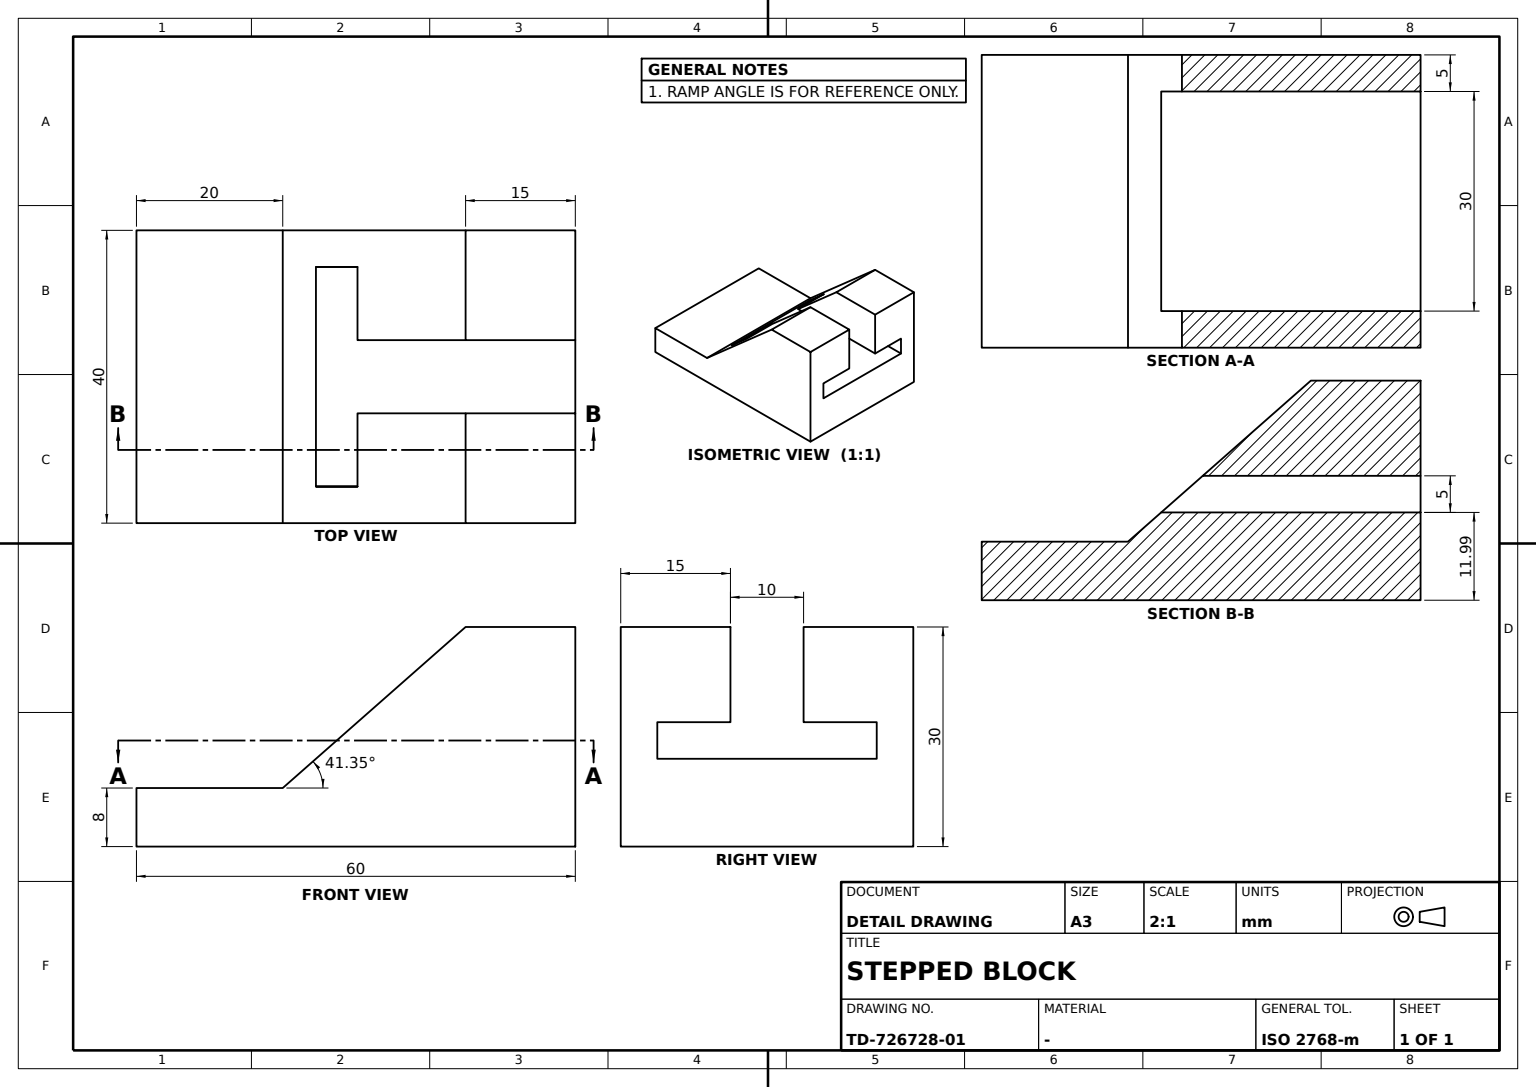
CATIA V5 part; units mm, degrees
sketch "Sketch1" plane through (0, 0, 0) normal (1, 0, 0) x (0, 1, 0)
  line L0 (0, 0) -> (0, 30)
  line L1 (0, 30) -> (-15, 30)
  line L2 (0, 0) -> (-60, 0)
  line L3 (-60, 0) -> (-60, 8)
  line L4 (-60, 8) -> (-40, 8)
  line L5 (-40, 8) -> (-15, 30)
  dimension "length L0" = 30
  dimension "length L1" = 15
  dimension "length L2" = 60
  dimension "length L3" = 8
  dimension "length L4" = 20
  constraint vertical L0 y-axis
  constraint vertical L3 y-axis
  constraint horizontal L1 x-axis
  constraint horizontal L2 x-axis
  constraint horizontal L4 x-axis
extrude "Pad1" add sketch "Sketch1" along normal mid plane 40
sketch "Sketch2" plane through (0, 0, 8) normal (0, 0, 1) x (0, 1, 0)
  line L0 (-65, -30) -> (-60, -30)
  line L1 (-60, -30) -> (-60, -50)
  line L2 (-60, -50) -> (-65, -50)
  line L3 (-65, -50) -> (-65, -30)
  line L4 (-60, 20) -> (-60, -20) construction
  line L5 (60, -20) -> (40, -20) construction
  dimension "length L0" = 5
  dimension "distance L0 L5" = 10
  dimension "length L3" = 20
  constraint horizontal L0 x-axis
  constraint horizontal L2 x-axis
  constraint vertical L1 y-axis
  constraint vertical L3 y-axis
  constraint coincidence L1 L4
extrude "Pocket1" cut sketch "Sketch2" against normal blind 20
sketch "Sketch3" plane through (0, -60, 0) normal (0, -1, 0) x (1, 0, 0)
  line L0 (-15, 11.9944) -> (15, 11.9944)
  line L1 (15, 11.9944) -> (15, 16.9944)
  line L2 (15, 16.9944) -> (5, 16.9944)
  line L3 (5, 16.9944) -> (5, 30.2766)
  line L4 (5, 30.2766) -> (-5, 30.2766)
  line L5 (-5, 30.2766) -> (-5, 16.9944)
  point P0 (-5, 16.9944)
  line L6 (-5, 16.9944) -> (-15, 16.9944)
  line L7 (-15, 16.9944) -> (-15, 11.9944)
  line L8 (-20, 30) -> (-20, 8) construction
  dimension "length L7" = 5
  dimension "length L0" = 30
  dimension "length L4" = 10
  dimension "distance L7 L8" = 5
  dimension "length L2" = 10
  constraint horizontal L0 x-axis
  constraint horizontal L2 x-axis
  constraint horizontal L4 x-axis
  constraint horizontal L6 x-axis
  constraint vertical L1 y-axis
  constraint vertical L3 y-axis
  constraint vertical L5 y-axis
  constraint vertical L7 y-axis
  constraint coincidence P0 L2
extrude "Pocket2" cut sketch "Sketch3" against normal through all
properties part number "catia 6"
